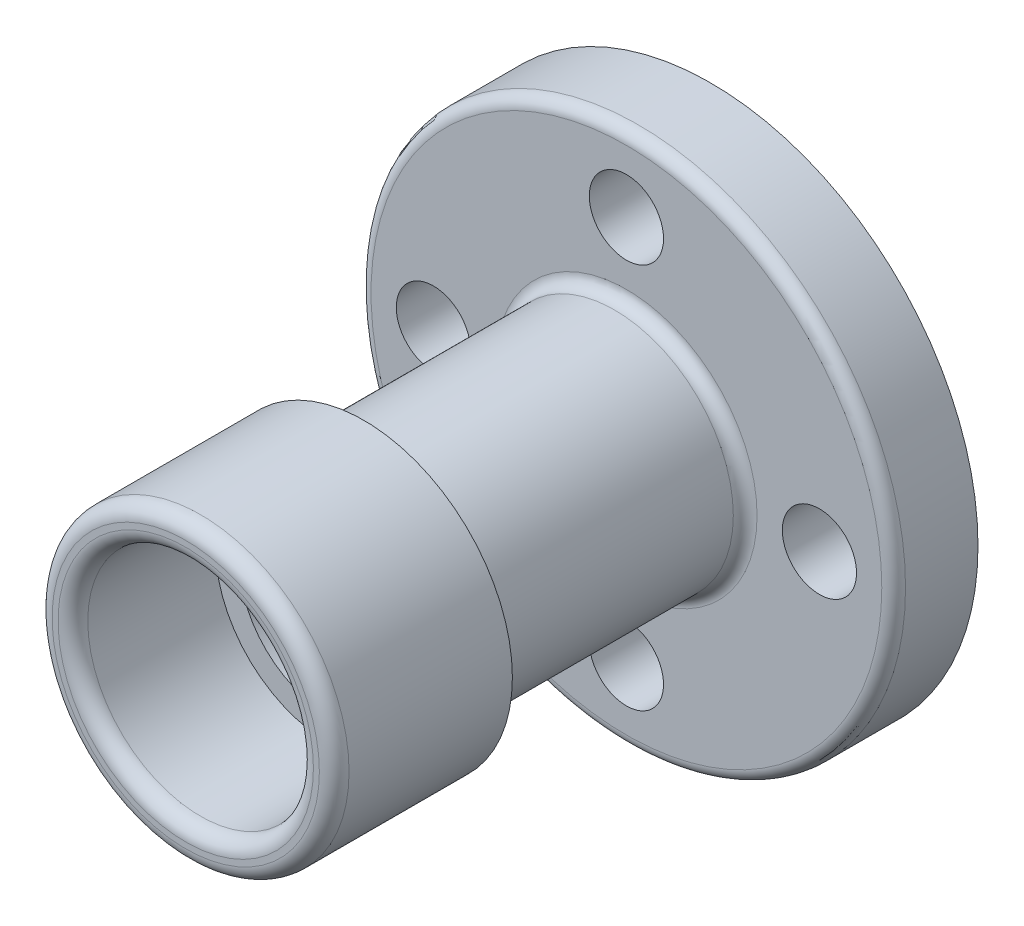
ISO-10303-21;
HEADER;
FILE_DESCRIPTION(('STEP AP214'),'2;1');
FILE_NAME('part.step','',(''),(''),'','','');
FILE_SCHEMA(('AUTOMOTIVE_DESIGN { 1 0 10303 214 1 1 1 1 }'));
ENDSEC;
DATA;
#1=APPLICATION_CONTEXT('core data for automotive mechanical design processes');
#2=APPLICATION_PROTOCOL_DEFINITION('international standard','automotive_design',2000,#1);
#3=PRODUCT_CONTEXT('',#1,'mechanical');
#4=PRODUCT('Part','Part','',(#3));
#5=PRODUCT_RELATED_PRODUCT_CATEGORY('part','',(#4));
#6=PRODUCT_DEFINITION_FORMATION('','',#4);
#7=PRODUCT_DEFINITION_CONTEXT('part definition',#1,'design');
#8=PRODUCT_DEFINITION('design','',#6,#7);
#9=PRODUCT_DEFINITION_SHAPE('','',#8);
#10=(LENGTH_UNIT() NAMED_UNIT(*) SI_UNIT(.MILLI.,.METRE.));
#11=(NAMED_UNIT(*) PLANE_ANGLE_UNIT() SI_UNIT($,.RADIAN.));
#12=(NAMED_UNIT(*) SI_UNIT($,.STERADIAN.) SOLID_ANGLE_UNIT());
#13=UNCERTAINTY_MEASURE_WITH_UNIT(LENGTH_MEASURE(1.E-05),#10,'distance_accuracy_value','');
#14=(GEOMETRIC_REPRESENTATION_CONTEXT(3) GLOBAL_UNCERTAINTY_ASSIGNED_CONTEXT((#13)) GLOBAL_UNIT_ASSIGNED_CONTEXT((#10,
#11,#12)) REPRESENTATION_CONTEXT('',''));
#15=CARTESIAN_POINT('',(0.,0.,0.));
#16=DIRECTION('',(0.,0.,1.));
#17=DIRECTION('',(1.,0.,0.));
#18=AXIS2_PLACEMENT_3D('',#15,#16,#17);
#19=CARTESIAN_POINT('',(0.,0.,64.4));
#20=DIRECTION('',(0.,0.,1.));
#21=DIRECTION('',(1.,0.,0.));
#22=AXIS2_PLACEMENT_3D('',#19,#20,#21);
#23=PLANE('',#22);
#24=CARTESIAN_POINT('',(0.,0.,64.4));
#25=DIRECTION('',(0.,0.,1.));
#26=DIRECTION('',(1.,0.,0.));
#27=AXIS2_PLACEMENT_3D('',#24,#25,#26);
#28=CIRCLE('',#27,15.);
#29=CARTESIAN_POINT('',(15.,0.,64.4));
#30=VERTEX_POINT('',#29);
#31=EDGE_CURVE('E109',#30,#30,#28,.T.);
#32=ORIENTED_EDGE('',*,*,#31,.F.);
#33=EDGE_LOOP('',(#32));
#34=FACE_BOUND('',#33,.T.);
#35=CARTESIAN_POINT('',(0.,0.,64.4));
#36=DIRECTION('',(0.,0.,1.));
#37=DIRECTION('',(1.,0.,0.));
#38=AXIS2_PLACEMENT_3D('',#35,#36,#37);
#39=CIRCLE('',#38,19.);
#40=CARTESIAN_POINT('',(19.,0.,64.4));
#41=VERTEX_POINT('',#40);
#42=EDGE_CURVE('E113',#41,#41,#39,.T.);
#43=ORIENTED_EDGE('',*,*,#42,.T.);
#44=EDGE_LOOP('',(#43));
#45=FACE_BOUND('',#44,.T.);
#46=ADVANCED_FACE('F39',(#34,#45),#23,.T.);
#47=CARTESIAN_POINT('',(0.,0.,14.2));
#48=DIRECTION('',(0.,0.,1.));
#49=DIRECTION('',(1.,0.,0.));
#50=AXIS2_PLACEMENT_3D('',#47,#48,#49);
#51=PLANE('',#50);
#52=CARTESIAN_POINT('',(0.,0.,14.2));
#53=DIRECTION('',(0.,0.,1.));
#54=DIRECTION('',(1.,0.,0.));
#55=AXIS2_PLACEMENT_3D('',#52,#53,#54);
#56=CIRCLE('',#55,22.);
#57=CARTESIAN_POINT('',(22.,0.,14.2));
#58=VERTEX_POINT('',#57);
#59=EDGE_CURVE('E56',#58,#58,#56,.F.);
#60=ORIENTED_EDGE('',*,*,#59,.T.);
#61=EDGE_LOOP('',(#60));
#62=FACE_BOUND('',#61,.T.);
#63=CARTESIAN_POINT('',(0.,-32.5,14.2));
#64=DIRECTION('',(0.,0.,1.));
#65=DIRECTION('',(-1.,0.,0.));
#66=AXIS2_PLACEMENT_3D('',#63,#64,#65);
#67=CIRCLE('',#66,6.25);
#68=CARTESIAN_POINT('',(-6.25,-32.5,14.2));
#69=VERTEX_POINT('',#68);
#70=EDGE_CURVE('E82',#69,#69,#67,.T.);
#71=ORIENTED_EDGE('',*,*,#70,.F.);
#72=EDGE_LOOP('',(#71));
#73=FACE_BOUND('',#72,.T.);
#74=CARTESIAN_POINT('',(32.5,0.,14.2));
#75=DIRECTION('',(0.,0.,1.));
#76=DIRECTION('',(-1.,0.,0.));
#77=AXIS2_PLACEMENT_3D('',#74,#75,#76);
#78=CIRCLE('',#77,6.25);
#79=CARTESIAN_POINT('',(26.25,0.,14.2));
#80=VERTEX_POINT('',#79);
#81=EDGE_CURVE('E90',#80,#80,#78,.T.);
#82=ORIENTED_EDGE('',*,*,#81,.F.);
#83=EDGE_LOOP('',(#82));
#84=FACE_BOUND('',#83,.T.);
#85=CARTESIAN_POINT('',(-32.5,0.,14.2));
#86=DIRECTION('',(0.,0.,1.));
#87=DIRECTION('',(1.,0.,0.));
#88=AXIS2_PLACEMENT_3D('',#85,#86,#87);
#89=CIRCLE('',#88,6.25);
#90=CARTESIAN_POINT('',(-26.25,0.,14.2));
#91=VERTEX_POINT('',#90);
#92=EDGE_CURVE('E93',#91,#91,#89,.T.);
#93=ORIENTED_EDGE('',*,*,#92,.F.);
#94=EDGE_LOOP('',(#93));
#95=FACE_BOUND('',#94,.T.);
#96=CARTESIAN_POINT('',(0.,32.5,14.2));
#97=DIRECTION('',(0.,0.,1.));
#98=DIRECTION('',(1.,0.,0.));
#99=AXIS2_PLACEMENT_3D('',#96,#97,#98);
#100=CIRCLE('',#99,6.25);
#101=CARTESIAN_POINT('',(6.25,32.5,14.2));
#102=VERTEX_POINT('',#101);
#103=EDGE_CURVE('E99',#102,#102,#100,.T.);
#104=ORIENTED_EDGE('',*,*,#103,.F.);
#105=EDGE_LOOP('',(#104));
#106=FACE_BOUND('',#105,.T.);
#107=CARTESIAN_POINT('',(0.,0.,14.2));
#108=DIRECTION('',(0.,0.,1.));
#109=DIRECTION('',(1.,0.,0.));
#110=AXIS2_PLACEMENT_3D('',#107,#108,#109);
#111=CIRCLE('',#110,43.);
#112=CARTESIAN_POINT('',(43.,0.,14.2));
#113=VERTEX_POINT('',#112);
#114=EDGE_CURVE('E73',#113,#113,#111,.T.);
#115=ORIENTED_EDGE('',*,*,#114,.T.);
#116=EDGE_LOOP('',(#115));
#117=FACE_BOUND('',#116,.T.);
#118=ADVANCED_FACE('F132',(#62,#73,#84,#95,#106,#117),#51,.T.);
#119=CARTESIAN_POINT('',(0.,0.,0.));
#120=DIRECTION('',(0.,0.,1.));
#121=DIRECTION('',(1.,0.,0.));
#122=AXIS2_PLACEMENT_3D('',#119,#120,#121);
#123=PLANE('',#122);
#124=CARTESIAN_POINT('',(0.,0.,0.));
#125=DIRECTION('',(0.,0.,1.));
#126=DIRECTION('',(1.,0.,0.));
#127=AXIS2_PLACEMENT_3D('',#124,#125,#126);
#128=CIRCLE('',#127,18.5);
#129=CARTESIAN_POINT('',(18.5,0.,0.));
#130=VERTEX_POINT('',#129);
#131=EDGE_CURVE('E70',#130,#130,#128,.T.);
#132=ORIENTED_EDGE('',*,*,#131,.T.);
#133=EDGE_LOOP('',(#132));
#134=FACE_BOUND('',#133,.T.);
#135=CARTESIAN_POINT('',(0.,32.5,0.));
#136=DIRECTION('',(0.,0.,1.));
#137=DIRECTION('',(1.,0.,0.));
#138=AXIS2_PLACEMENT_3D('',#135,#136,#137);
#139=CIRCLE('',#138,6.25);
#140=CARTESIAN_POINT('',(6.25,32.5,0.));
#141=VERTEX_POINT('',#140);
#142=EDGE_CURVE('E78',#141,#141,#139,.T.);
#143=ORIENTED_EDGE('',*,*,#142,.T.);
#144=EDGE_LOOP('',(#143));
#145=FACE_BOUND('',#144,.T.);
#146=CARTESIAN_POINT('',(-32.5,0.,0.));
#147=DIRECTION('',(0.,0.,1.));
#148=DIRECTION('',(1.,0.,0.));
#149=AXIS2_PLACEMENT_3D('',#146,#147,#148);
#150=CIRCLE('',#149,6.25);
#151=CARTESIAN_POINT('',(-26.25,0.,0.));
#152=VERTEX_POINT('',#151);
#153=EDGE_CURVE('E97',#152,#152,#150,.T.);
#154=ORIENTED_EDGE('',*,*,#153,.T.);
#155=EDGE_LOOP('',(#154));
#156=FACE_BOUND('',#155,.T.);
#157=CARTESIAN_POINT('',(32.5,0.,0.));
#158=DIRECTION('',(0.,0.,1.));
#159=DIRECTION('',(-1.,0.,0.));
#160=AXIS2_PLACEMENT_3D('',#157,#158,#159);
#161=CIRCLE('',#160,6.25);
#162=CARTESIAN_POINT('',(26.25,0.,0.));
#163=VERTEX_POINT('',#162);
#164=EDGE_CURVE('E91',#163,#163,#161,.T.);
#165=ORIENTED_EDGE('',*,*,#164,.T.);
#166=EDGE_LOOP('',(#165));
#167=FACE_BOUND('',#166,.T.);
#168=CARTESIAN_POINT('',(0.,-32.5,0.));
#169=DIRECTION('',(0.,0.,1.));
#170=DIRECTION('',(-1.,0.,0.));
#171=AXIS2_PLACEMENT_3D('',#168,#169,#170);
#172=CIRCLE('',#171,6.25);
#173=CARTESIAN_POINT('',(-6.25,-32.5,0.));
#174=VERTEX_POINT('',#173);
#175=EDGE_CURVE('E81',#174,#174,#172,.T.);
#176=ORIENTED_EDGE('',*,*,#175,.T.);
#177=EDGE_LOOP('',(#176));
#178=FACE_BOUND('',#177,.T.);
#179=CARTESIAN_POINT('',(0.,0.,0.));
#180=DIRECTION('',(0.,0.,1.));
#181=DIRECTION('',(1.,0.,0.));
#182=AXIS2_PLACEMENT_3D('',#179,#180,#181);
#183=CIRCLE('',#182,45.);
#184=CARTESIAN_POINT('',(45.,0.,0.));
#185=VERTEX_POINT('',#184);
#186=EDGE_CURVE('E80',#185,#185,#183,.T.);
#187=ORIENTED_EDGE('',*,*,#186,.F.);
#188=EDGE_LOOP('',(#187));
#189=FACE_BOUND('',#188,.T.);
#190=ADVANCED_FACE('F141',(#134,#145,#156,#167,#178,#189),#123,.F.);
#191=CARTESIAN_POINT('',(0.,0.,14.2));
#192=DIRECTION('',(0.,0.,-1.));
#193=DIRECTION('',(-1.,0.,0.));
#194=AXIS2_PLACEMENT_3D('',#191,#192,#193);
#195=CYLINDRICAL_SURFACE('',#194,45.);
#196=CARTESIAN_POINT('',(0.,0.,12.2));
#197=DIRECTION('',(0.,0.,1.));
#198=DIRECTION('',(1.,0.,0.));
#199=AXIS2_PLACEMENT_3D('',#196,#197,#198);
#200=CIRCLE('',#199,45.);
#201=CARTESIAN_POINT('',(45.,0.,12.2));
#202=VERTEX_POINT('',#201);
#203=EDGE_CURVE('E71',#202,#202,#200,.F.);
#204=ORIENTED_EDGE('',*,*,#203,.T.);
#205=EDGE_LOOP('',(#204));
#206=FACE_BOUND('',#205,.T.);
#207=ORIENTED_EDGE('',*,*,#186,.T.);
#208=EDGE_LOOP('',(#207));
#209=FACE_BOUND('',#208,.T.);
#210=ADVANCED_FACE('F176',(#206,#209),#195,.T.);
#211=CARTESIAN_POINT('',(0.,0.,14.2));
#212=DIRECTION('',(0.,0.,-1.));
#213=DIRECTION('',(-1.,0.,0.));
#214=AXIS2_PLACEMENT_3D('',#211,#212,#213);
#215=CYLINDRICAL_SURFACE('',#214,15.);
#216=CARTESIAN_POINT('',(0.,0.,3.00000000000003));
#217=DIRECTION('',(0.,0.,1.));
#218=DIRECTION('',(1.,0.,0.));
#219=AXIS2_PLACEMENT_3D('',#216,#217,#218);
#220=CIRCLE('',#219,15.);
#221=CARTESIAN_POINT('',(15.,0.,3.00000000000003));
#222=VERTEX_POINT('',#221);
#223=EDGE_CURVE('E63',#222,#222,#220,.F.);
#224=ORIENTED_EDGE('',*,*,#223,.T.);
#225=EDGE_LOOP('',(#224));
#226=FACE_BOUND('',#225,.T.);
#227=ORIENTED_EDGE('',*,*,#31,.T.);
#228=EDGE_LOOP('',(#227));
#229=FACE_BOUND('',#228,.T.);
#230=ADVANCED_FACE('F173',(#226,#229),#215,.F.);
#231=CARTESIAN_POINT('',(0.,-32.5,0.));
#232=DIRECTION('',(0.,0.,1.));
#233=DIRECTION('',(1.,0.,0.));
#234=AXIS2_PLACEMENT_3D('',#231,#232,#233);
#235=CYLINDRICAL_SURFACE('',#234,6.25);
#236=ORIENTED_EDGE('',*,*,#175,.F.);
#237=EDGE_LOOP('',(#236));
#238=FACE_BOUND('',#237,.T.);
#239=ORIENTED_EDGE('',*,*,#70,.T.);
#240=EDGE_LOOP('',(#239));
#241=FACE_BOUND('',#240,.T.);
#242=ADVANCED_FACE('F169',(#238,#241),#235,.F.);
#243=CARTESIAN_POINT('',(32.5,0.,0.));
#244=DIRECTION('',(0.,0.,1.));
#245=DIRECTION('',(1.,0.,0.));
#246=AXIS2_PLACEMENT_3D('',#243,#244,#245);
#247=CYLINDRICAL_SURFACE('',#246,6.25);
#248=ORIENTED_EDGE('',*,*,#164,.F.);
#249=EDGE_LOOP('',(#248));
#250=FACE_BOUND('',#249,.T.);
#251=ORIENTED_EDGE('',*,*,#81,.T.);
#252=EDGE_LOOP('',(#251));
#253=FACE_BOUND('',#252,.T.);
#254=ADVANCED_FACE('F164',(#250,#253),#247,.F.);
#255=CARTESIAN_POINT('',(-32.5,0.,0.));
#256=DIRECTION('',(0.,0.,1.));
#257=DIRECTION('',(1.,0.,0.));
#258=AXIS2_PLACEMENT_3D('',#255,#256,#257);
#259=CYLINDRICAL_SURFACE('',#258,6.25);
#260=ORIENTED_EDGE('',*,*,#153,.F.);
#261=EDGE_LOOP('',(#260));
#262=FACE_BOUND('',#261,.T.);
#263=ORIENTED_EDGE('',*,*,#92,.T.);
#264=EDGE_LOOP('',(#263));
#265=FACE_BOUND('',#264,.T.);
#266=ADVANCED_FACE('F163',(#262,#265),#259,.F.);
#267=CARTESIAN_POINT('',(0.,32.5,0.));
#268=DIRECTION('',(0.,0.,1.));
#269=DIRECTION('',(1.,0.,0.));
#270=AXIS2_PLACEMENT_3D('',#267,#268,#269);
#271=CYLINDRICAL_SURFACE('',#270,6.25);
#272=ORIENTED_EDGE('',*,*,#142,.F.);
#273=EDGE_LOOP('',(#272));
#274=FACE_BOUND('',#273,.T.);
#275=ORIENTED_EDGE('',*,*,#103,.T.);
#276=EDGE_LOOP('',(#275));
#277=FACE_BOUND('',#276,.T.);
#278=ADVANCED_FACE('F157',(#274,#277),#271,.F.);
#279=CARTESIAN_POINT('',(0.,0.,12.2));
#280=DIRECTION('',(0.,0.,1.));
#281=DIRECTION('',(1.,0.,0.));
#282=AXIS2_PLACEMENT_3D('',#279,#280,#281);
#283=TOROIDAL_SURFACE('',#282,43.,2.);
#284=ORIENTED_EDGE('',*,*,#203,.F.);
#285=EDGE_LOOP('',(#284));
#286=FACE_BOUND('',#285,.T.);
#287=ORIENTED_EDGE('',*,*,#114,.F.);
#288=EDGE_LOOP('',(#287));
#289=FACE_BOUND('',#288,.T.);
#290=ADVANCED_FACE('F156',(#286,#289),#283,.T.);
#291=CARTESIAN_POINT('',(0.,0.,58.4));
#292=DIRECTION('',(0.,0.,-1.));
#293=DIRECTION('',(-1.,0.,0.));
#294=AXIS2_PLACEMENT_3D('',#291,#292,#293);
#295=CYLINDRICAL_SURFACE('',#294,20.);
#296=CARTESIAN_POINT('',(0.,0.,16.2));
#297=DIRECTION('',(0.,0.,1.));
#298=DIRECTION('',(1.,0.,0.));
#299=AXIS2_PLACEMENT_3D('',#296,#297,#298);
#300=CIRCLE('',#299,20.);
#301=CARTESIAN_POINT('',(20.,0.,16.2));
#302=VERTEX_POINT('',#301);
#303=EDGE_CURVE('E65',#302,#302,#300,.T.);
#304=ORIENTED_EDGE('',*,*,#303,.T.);
#305=EDGE_LOOP('',(#304));
#306=FACE_BOUND('',#305,.T.);
#307=CARTESIAN_POINT('',(0.,0.,58.4));
#308=DIRECTION('',(0.,0.,1.));
#309=DIRECTION('',(1.,0.,0.));
#310=AXIS2_PLACEMENT_3D('',#307,#308,#309);
#311=CIRCLE('',#310,20.);
#312=CARTESIAN_POINT('',(20.,0.,58.4));
#313=VERTEX_POINT('',#312);
#314=EDGE_CURVE('E83',#313,#313,#311,.T.);
#315=ORIENTED_EDGE('',*,*,#314,.F.);
#316=EDGE_LOOP('',(#315));
#317=FACE_BOUND('',#316,.T.);
#318=ADVANCED_FACE('F148',(#306,#317),#295,.T.);
#319=CARTESIAN_POINT('',(0.,0.,58.4));
#320=DIRECTION('',(0.,0.,1.));
#321=DIRECTION('',(1.,0.,0.));
#322=AXIS2_PLACEMENT_3D('',#319,#320,#321);
#323=PLANE('',#322);
#324=ORIENTED_EDGE('',*,*,#314,.T.);
#325=EDGE_LOOP('',(#324));
#326=FACE_BOUND('',#325,.T.);
#327=CARTESIAN_POINT('',(0.,0.,58.4));
#328=DIRECTION('',(0.,0.,1.));
#329=DIRECTION('',(1.,0.,0.));
#330=AXIS2_PLACEMENT_3D('',#327,#328,#329);
#331=CIRCLE('',#330,25.);
#332=CARTESIAN_POINT('',(25.,0.,58.4));
#333=VERTEX_POINT('',#332);
#334=EDGE_CURVE('E110',#333,#333,#331,.T.);
#335=ORIENTED_EDGE('',*,*,#334,.F.);
#336=EDGE_LOOP('',(#335));
#337=FACE_BOUND('',#336,.T.);
#338=ADVANCED_FACE('F149',(#326,#337),#323,.F.);
#339=CARTESIAN_POINT('',(0.,0.,64.4));
#340=DIRECTION('',(0.,0.,-1.));
#341=DIRECTION('',(-1.,0.,0.));
#342=AXIS2_PLACEMENT_3D('',#339,#340,#341);
#343=CYLINDRICAL_SURFACE('',#342,25.);
#344=CARTESIAN_POINT('',(0.,0.,85.9));
#345=DIRECTION('',(0.,0.,1.));
#346=DIRECTION('',(1.,0.,0.));
#347=AXIS2_PLACEMENT_3D('',#344,#345,#346);
#348=CIRCLE('',#347,25.);
#349=CARTESIAN_POINT('',(25.,0.,85.9));
#350=VERTEX_POINT('',#349);
#351=EDGE_CURVE('E10',#350,#350,#348,.F.);
#352=ORIENTED_EDGE('',*,*,#351,.T.);
#353=EDGE_LOOP('',(#352));
#354=FACE_BOUND('',#353,.T.);
#355=ORIENTED_EDGE('',*,*,#334,.T.);
#356=EDGE_LOOP('',(#355));
#357=FACE_BOUND('',#356,.T.);
#358=ADVANCED_FACE('F131',(#354,#357),#343,.T.);
#359=CARTESIAN_POINT('',(0.,0.,88.4));
#360=DIRECTION('',(0.,0.,1.));
#361=DIRECTION('',(1.,0.,0.));
#362=AXIS2_PLACEMENT_3D('',#359,#360,#361);
#363=PLANE('',#362);
#364=CARTESIAN_POINT('',(0.,0.,88.4));
#365=DIRECTION('',(0.,0.,1.));
#366=DIRECTION('',(1.,0.,0.));
#367=AXIS2_PLACEMENT_3D('',#364,#365,#366);
#368=CIRCLE('',#367,21.5);
#369=CARTESIAN_POINT('',(21.5,0.,88.4));
#370=VERTEX_POINT('',#369);
#371=EDGE_CURVE('E46',#370,#370,#368,.F.);
#372=ORIENTED_EDGE('',*,*,#371,.T.);
#373=EDGE_LOOP('',(#372));
#374=FACE_BOUND('',#373,.T.);
#375=CARTESIAN_POINT('',(0.,0.,88.4));
#376=DIRECTION('',(0.,0.,1.));
#377=DIRECTION('',(1.,0.,0.));
#378=AXIS2_PLACEMENT_3D('',#375,#376,#377);
#379=CIRCLE('',#378,22.5);
#380=CARTESIAN_POINT('',(22.5,0.,88.4));
#381=VERTEX_POINT('',#380);
#382=EDGE_CURVE('E49',#381,#381,#379,.T.);
#383=ORIENTED_EDGE('',*,*,#382,.T.);
#384=EDGE_LOOP('',(#383));
#385=FACE_BOUND('',#384,.T.);
#386=ADVANCED_FACE('F122',(#374,#385),#363,.T.);
#387=CARTESIAN_POINT('',(0.,0.,88.4));
#388=DIRECTION('',(0.,0.,-1.));
#389=DIRECTION('',(-1.,0.,0.));
#390=AXIS2_PLACEMENT_3D('',#387,#388,#389);
#391=CYLINDRICAL_SURFACE('',#390,19.);
#392=CARTESIAN_POINT('',(0.,0.,85.9));
#393=DIRECTION('',(0.,0.,1.));
#394=DIRECTION('',(1.,0.,0.));
#395=AXIS2_PLACEMENT_3D('',#392,#393,#394);
#396=CIRCLE('',#395,19.);
#397=CARTESIAN_POINT('',(19.,0.,85.9));
#398=VERTEX_POINT('',#397);
#399=EDGE_CURVE('E53',#398,#398,#396,.T.);
#400=ORIENTED_EDGE('',*,*,#399,.T.);
#401=EDGE_LOOP('',(#400));
#402=FACE_BOUND('',#401,.T.);
#403=ORIENTED_EDGE('',*,*,#42,.F.);
#404=EDGE_LOOP('',(#403));
#405=FACE_BOUND('',#404,.T.);
#406=ADVANCED_FACE('F117',(#402,#405),#391,.F.);
#407=CARTESIAN_POINT('',(0.,0.,0.));
#408=DIRECTION('',(0.,0.,-1.));
#409=DIRECTION('',(-1.,0.,0.));
#410=AXIS2_PLACEMENT_3D('',#407,#408,#409);
#411=CONICAL_SURFACE('',#410,18.5,0.862170054667228);
#412=ORIENTED_EDGE('',*,*,#223,.F.);
#413=EDGE_LOOP('',(#412));
#414=FACE_BOUND('',#413,.T.);
#415=ORIENTED_EDGE('',*,*,#131,.F.);
#416=EDGE_LOOP('',(#415));
#417=FACE_BOUND('',#416,.T.);
#418=ADVANCED_FACE('F119',(#414,#417),#411,.F.);
#419=CARTESIAN_POINT('',(0.,0.,16.2));
#420=DIRECTION('',(0.,0.,1.));
#421=DIRECTION('',(1.,0.,0.));
#422=AXIS2_PLACEMENT_3D('',#419,#420,#421);
#423=TOROIDAL_SURFACE('',#422,22.,2.);
#424=ORIENTED_EDGE('',*,*,#59,.F.);
#425=EDGE_LOOP('',(#424));
#426=FACE_BOUND('',#425,.T.);
#427=ORIENTED_EDGE('',*,*,#303,.F.);
#428=EDGE_LOOP('',(#427));
#429=FACE_BOUND('',#428,.T.);
#430=ADVANCED_FACE('F126',(#426,#429),#423,.F.);
#431=CARTESIAN_POINT('',(0.,0.,85.9));
#432=DIRECTION('',(0.,0.,1.));
#433=DIRECTION('',(1.,0.,0.));
#434=AXIS2_PLACEMENT_3D('',#431,#432,#433);
#435=TOROIDAL_SURFACE('',#434,21.5,2.5);
#436=ORIENTED_EDGE('',*,*,#371,.F.);
#437=EDGE_LOOP('',(#436));
#438=FACE_BOUND('',#437,.T.);
#439=ORIENTED_EDGE('',*,*,#399,.F.);
#440=EDGE_LOOP('',(#439));
#441=FACE_BOUND('',#440,.T.);
#442=ADVANCED_FACE('F192',(#438,#441),#435,.T.);
#443=CARTESIAN_POINT('',(0.,0.,85.9));
#444=DIRECTION('',(0.,0.,1.));
#445=DIRECTION('',(1.,0.,0.));
#446=AXIS2_PLACEMENT_3D('',#443,#444,#445);
#447=TOROIDAL_SURFACE('',#446,22.5,2.5);
#448=ORIENTED_EDGE('',*,*,#351,.F.);
#449=EDGE_LOOP('',(#448));
#450=FACE_BOUND('',#449,.T.);
#451=ORIENTED_EDGE('',*,*,#382,.F.);
#452=EDGE_LOOP('',(#451));
#453=FACE_BOUND('',#452,.T.);
#454=ADVANCED_FACE('F41',(#450,#453),#447,.T.);
#455=CLOSED_SHELL('',(#46,#118,#190,#210,#230,#242,#254,#266,#278,#290,#318,#338,#358,#386,#406,
#418,#430,#442,#454));
#456=MANIFOLD_SOLID_BREP('B2',#455);
#457=ADVANCED_BREP_SHAPE_REPRESENTATION('',(#18,#456),#14);
#458=SHAPE_DEFINITION_REPRESENTATION(#9,#457);
ENDSEC;
END-ISO-10303-21;
